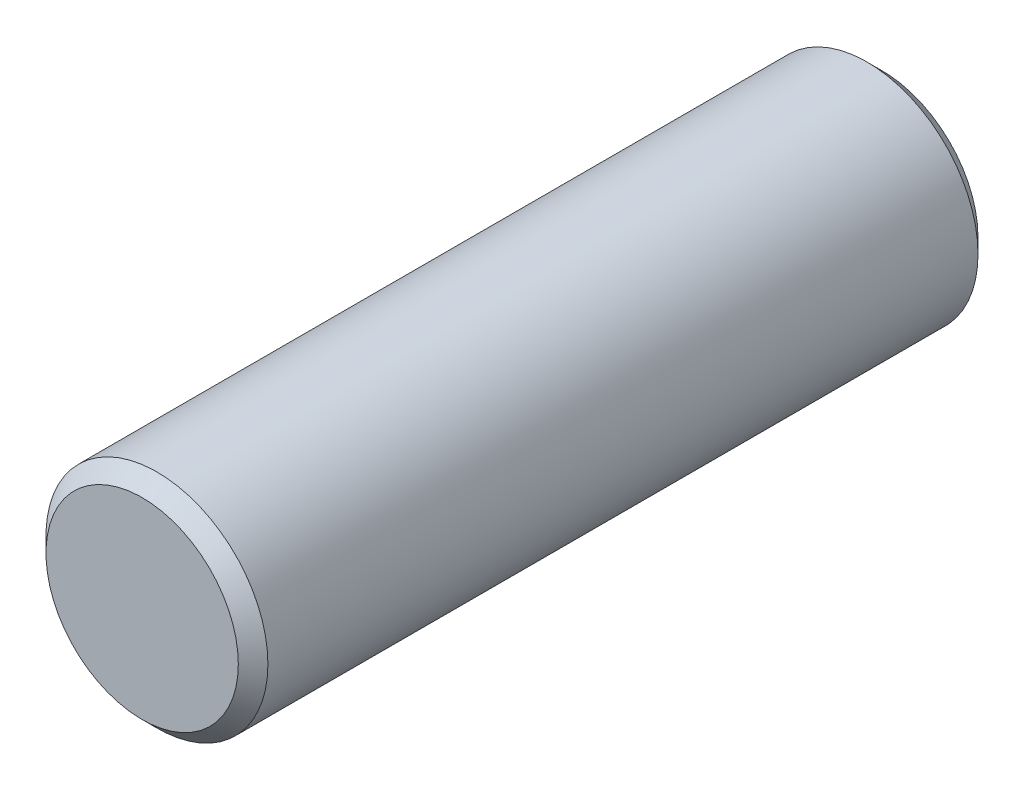
SolidWorks part; units mm, degrees
material "Plain Carbon Steel"
ref_plane "Front Plane" through (0, 0, 0) normal (0, 0, 1) x (1, 0, 0)
ref_plane "Top Plane" through (0, 0, 0) normal (0, 1, 0) x (1, 0, 0)
ref_plane "Right Plane" through (0, 0, 0) normal (1, 0, 0) x (0, 0, -1)
sketch "Pin Profile Ø3" plane through (0, 0, 0) normal (0, 0, 1) x (1, 0, 0)
  circle A0 centre (0, 0) radius 1.5
  dimension "D1" = 3
extrude "Pin Body Ø3x10" add sketch "Pin Profile Ø3" along normal mid plane 10
chamfer "End Chamfers 0.2x45°" distance 0.2 angle 45 2 edges at (1.5, 0, -5) (1.5, 0, 5)
